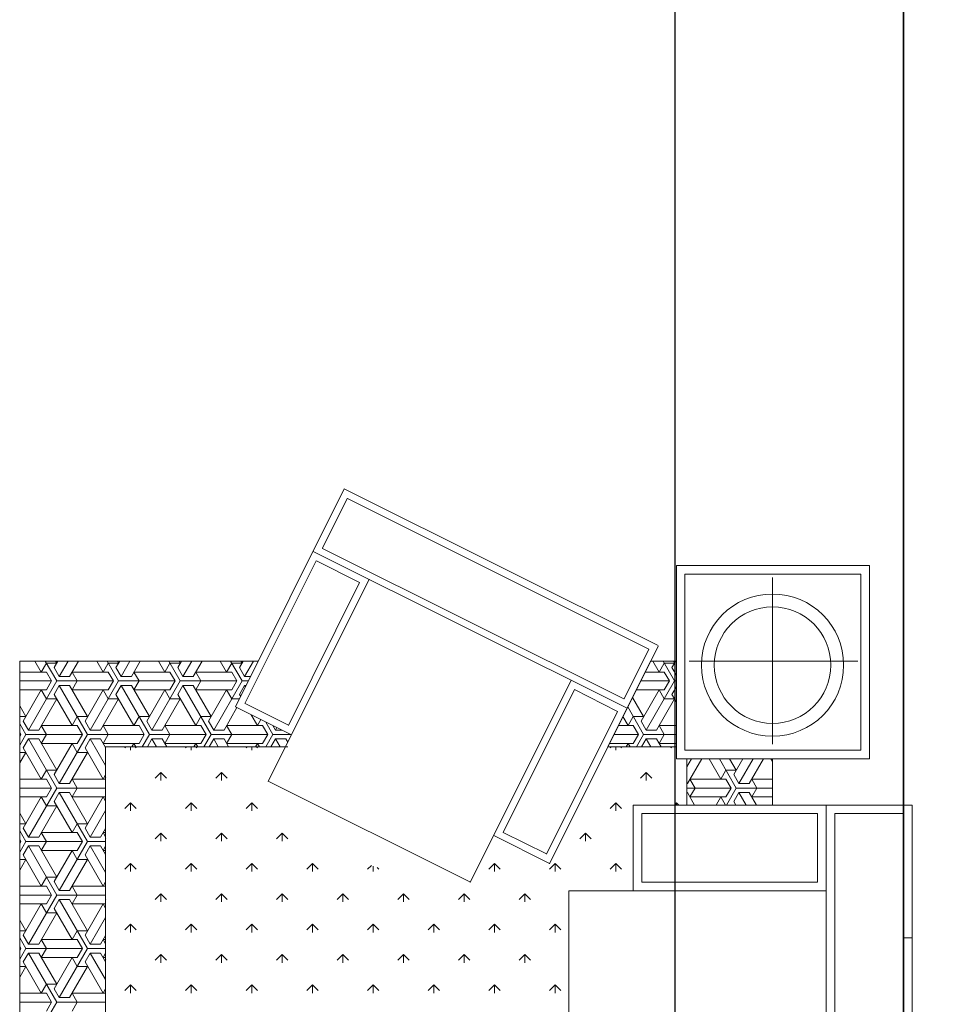
# Model space of a CAD drawing. Units: inches. Extents: x -1198 to -69, y -512 to 437.
# Tile 23 of 50: x -750 to -696, y 76 to 134. Entities that reach past the tile are written whole.
import ezdxf

# ---------------------------------------------------------------- set-up
doc = ezdxf.new("R2010")
doc.units = ezdxf.units.IN
doc.header["$MEASUREMENT"] = 0
for name, color, linetype, lineweight in [('A-ANNO-DIMS', 2, 'Continuous', 18), ('A-FURN', 60, 'Continuous', 18), ('A-WALL', 7, 'Continuous', 35), ('windows', 160, 'Continuous', 18)]:
    doc.layers.add(name, color=color, linetype=linetype, lineweight=lineweight)
doc.styles.get("Standard").update_dxf_attribs({"font": 'arial.ttf'})
doc.dimstyles.get("Standard").update_dxf_attribs({"dimtxt": 6, "dimasz": 6, "dimexe": 0.18, "dimexo": 0.0625, "dimgap": 0.09, "dimtad": 0, "dimtih": 1, "dimtoh": 1, "dimdec": 0, "dimzin": 0, "dimdsep": 46, "dimlunit": 4, "dimtxsty": 'Standard', "dimblk": 'OBLIQUE', "dimcen": 0.09, "dimadec": 0, "dimazin": 0, "dimtfac": 1, "dimtdec": 0, "dimtofl": 0, "dimtmove": 0, "dimatfit": 3, "dimfxl": 1, "dimtolj": 1, "dimtzin": 0, "dimarcsym": 0})

# ---------------------------------------------------------------- blocks, each defined once
blk = doc.blocks.new('A$C3B9F700E')
for p, q in [((736.9, 2080, -685.7), (2936.9, 2080, -685.7)), ((736.9, 2080, -685.7), (736.9, 1430, -685.7)), ((736.9, 1880, -685.7), (736.9, 2080, -685.7)), ((756.9, 2060, -685.7), (2916.9, 2060, -685.7)), ((756.9, 1900, -685.7), (756.9, 2060, -685.7)), ((179, 1980.6, -685.7), (179, 1530.6, -685.7)), ((629, 1980.6, -685.7), (179, 1980.6, -685.7)), ((629, 1530.6, -685.7), (629, 1980.6, -685.7)), ((199, 1960.6, -685.7), (199, 1550.6, -685.7)), ((609, 1960.6, -685.7), (199, 1960.6, -685.7)), ((401.3, 1953.9, -685.7), (401.3, 1560.5, -685.7)), ((609, 1550.6, -685.7), (609, 1960.6, -685.7)), ((2916.9, 1900, -685.7), (756.9, 1900, -685.7)), ((2936.9, 1880, -685.7), (736.9, 1880, -685.7)), ((2936.9, 1880, -685.7), (736.9, 1880, -685.7)), ((736.9, 1430, -685.7), (736.9, 1880, -685.7)), ((736.9, 1880, -685.7), (936.9, 1880, -685.7)), ((756.9, 1450, -685.7), (756.9, 1860, -685.7)), ((756.9, 1860, -685.7), (916.9, 1860, -685.7)), ((916.9, 1860, -685.7), (916.9, 1450, -685.7)), ((936.9, 1880, -685.7), (936.9, 1280, -685.7)), ((936.9, 1880, -685.7), (936.9, 1430, -685.7)), ((595.4, 1754.8, -685.7), (207.1, 1754.8, -685.7)), ((629, 1754.8, -685.7), (736.9, 1754.8, -685.7)), ((629, 1754.8, -685.7), (736.9, 1754.8, -685.7)), ((629, 1554.8, -685.7), (629, 1754.8, -685.7)), ((629, 1750.9, -685.7), (635.7, 1754.8, -685.7)), ((676.4, 1754.8, -685.7), (676.4, 1706.3, -685.7)), ((697.2, 1670.3, -685.7), (697.2, 1754.8, -685.7)), ((718, 1754.8, -685.7), (718, 1706.3, -685.7)), ((736.9, 1754.8, -685.7), (736.9, 1554.8, -685.7)), ((686.8, 1700.3, -685.7), (629, 1733.7, -685.7)), ((629, 1709.7, -685.7), (686.8, 1676.3, -685.7)), ((697.2, 1718.3, -685.7), (676.4, 1706.3, -685.7)), ((686.8, 1676.3, -685.7), (686.8, 1700.3, -685.7)), ((697.2, 1718.3, -685.7), (718, 1706.3, -685.7)), ((707.6, 1700.3, -685.7), (736.9, 1717.3, -685.7)), ((707.6, 1676.3, -685.7), (707.6, 1700.3, -685.7)), ((666, 1664.3, -685.7), (629, 1685.7, -685.7)), ((686.8, 1676.3, -685.7), (666, 1664.3, -685.7)), ((736.9, 1693.3, -685.7), (707.6, 1676.3, -685.7)), ((707.6, 1676.3, -685.7), (728.4, 1664.3, -685.7)), ((629, 1654.9, -685.7), (655.6, 1670.3, -685.7)), ((697.2, 1670.3, -685.7), (629, 1630.9, -685.7)), ((655.6, 1646.3, -685.7), (655.6, 1670.3, -685.7)), ((697.2, 1658.3, -685.7), (676.4, 1646.3, -685.7)), ((697.2, 1670.3, -685.7), (736.9, 1647.4, -685.7)), ((697.2, 1658.3, -685.7), (718, 1646.3, -685.7)), ((697.2, 1554.8, -685.7), (697.2, 1658.3, -685.7)), ((728.4, 1664.3, -685.7), (736.9, 1669.3, -685.7)), ((629, 1606.9, -685.7), (676.4, 1634.3, -685.7)), ((655.6, 1646.3, -685.7), (676.4, 1634.3, -685.7)), ((676.4, 1646.3, -685.7), (676.4, 1562.3, -685.7)), ((718, 1646.3, -685.7), (718, 1562.3, -685.7)), ((736.9, 1645.3, -685.7), (718, 1634.3, -685.7)), ((736.9, 1623.4, -685.7), (718, 1634.3, -685.7)), ((686.8, 1556.3, -685.7), (629, 1589.7, -685.7)), ((629, 1565.7, -685.7), (647.9, 1554.8, -685.7)), ((697.2, 1574.3, -685.7), (676.4, 1562.3, -685.7)), ((697.2, 1574.3, -685.7), (718, 1562.3, -685.7)), ((707.6, 1556.3, -685.7), (736.9, 1573.3, -685.7)), ((199, 1550.6, -685.7), (609, 1550.6, -685.7)), ((736.9, 1554.8, -685.7), (629, 1554.8, -685.7)), ((629, 1554.8, -685.7), (736.9, 1554.8, -685.7)), ((686.8, 1554.8, -685.7), (686.8, 1556.3, -685.7)), ((707.6, 1554.8, -685.7), (707.6, 1556.3, -685.7)), ((179, 1530.6, -685.7), (629, 1530.6, -685.7)), ((401.4, 1530.6, -685.7), (401.4, 1470.6, -685.7)), ((401.4, 1470.6, -685.7), (401.4, 1530.6, -685.7)), ((601.4, 1530.6, -685.7), (401.4, 1530.6, -685.7)), ((416.6, 1520.3, -685.7), (401.4, 1529.1, -685.7)), ((401.4, 1523.6, -685.7), (406.2, 1526.3, -685.7)), ((447.8, 1526.3, -685.7), (401.4, 1499.6, -685.7)), ((406.2, 1502.3, -685.7), (406.2, 1526.3, -685.7)), ((434.4, 1530.6, -685.7), (416.6, 1520.3, -685.7)), ((447.8, 1514.3, -685.7), (427, 1502.3, -685.7)), ((447.8, 1526.3, -685.7), (447.8, 1530.6, -685.7)), ((447.8, 1526.3, -685.7), (562.1, 1460.3, -685.7)), ((447.8, 1514.3, -685.7), (468.6, 1502.3, -685.7)), ((447.8, 1447.5, -685.7), (447.8, 1514.3, -685.7)), ((461.1, 1530.6, -685.7), (479, 1520.3, -685.7)), ((479, 1520.3, -685.7), (496.8, 1530.6, -685.7)), ((562.1, 1484.3, -685.7), (489.3, 1526.3, -685.7)), ((489.3, 1502.3, -685.7), (489.3, 1526.3, -685.7)), ((551.7, 1530.6, -685.7), (551.7, 1490.3, -685.7)), ((572.5, 1454.3, -685.7), (572.5, 1530.6, -685.7)), ((593.3, 1530.6, -685.7), (593.3, 1490.3, -685.7)), ((601.4, 1370.8, -685.7), (601.4, 1530.6, -685.7)), ((601.4, 1370.8, -685.7), (601.4, 1530.6, -685.7)), ((601.4, 1520.3, -685.7), (603.7, 1518, -685.7)), ((731.9, 1531.3, -685.7), (736.9, 1536.3, -685.7)), ((731.9, 1531.3, -685.7), (736.9, 1526.2, -685.7)), ((731.9, 1531.3, -685.7), (736.9, 1531.3, -685.7)), ((406.2, 1502.3, -685.7), (427, 1490.3, -685.7)), ((427, 1502.3, -685.7), (427, 1457.9, -685.7)), ((468.6, 1502.3, -685.7), (468.6, 1437.1, -685.7)), ((489.3, 1502.3, -685.7), (468.6, 1490.3, -685.7)), ((572.5, 1502.3, -685.7), (551.7, 1490.3, -685.7)), ((572.5, 1502.3, -685.7), (593.3, 1490.3, -685.7)), ((582.9, 1484.3, -685.7), (601.4, 1495, -685.7)), ((365.5, 1488.6, -685.7), (0, 756.7, -685.7)), ((873.7, 1234.8, -685.7), (366.4, 1488.1, -685.7)), ((401.4, 1475.6, -685.7), (427, 1490.3, -685.7)), ((401.4, 1470.6, -685.7), (601.4, 1370.8, -685.7)), ((541.3, 1448.3, -685.7), (468.6, 1490.3, -685.7)), ((562.1, 1460.3, -685.7), (562.1, 1484.3, -685.7)), ((582.9, 1460.3, -685.7), (582.9, 1484.3, -685.7)), ((601.4, 1471, -685.7), (582.9, 1460.3, -685.7)), ((661.2, 1460.6, -685.7), (674.4, 1473.8, -685.7)), ((373.6, 1466.4, -685.7), (22.8, 763.8, -685.7)), ((489.2, 1408.7, -685.7), (373.6, 1466.4, -685.7)), ((486, 1428.4, -685.7), (530.9, 1454.3, -685.7)), ((572.5, 1454.3, -685.7), (508.3, 1417.3, -685.7)), ((530.9, 1430.3, -685.7), (530.9, 1454.3, -685.7)), ((562.1, 1460.3, -685.7), (541.3, 1448.3, -685.7)), ((572.5, 1454.3, -685.7), (601.4, 1437.6, -685.7)), ((582.9, 1460.3, -685.7), (601.4, 1449.6, -685.7)), ((661.2, 1460.6, -685.7), (674.4, 1447.3, -685.7)), ((661.2, 1460.6, -685.7), (679.9, 1460.6, -685.7)), ((916.9, 1450, -685.7), (756.9, 1450, -685.7)), ((530.9, 1430.3, -685.7), (551.7, 1418.3, -685.7)), ((572.5, 1442.3, -685.7), (551.7, 1430.3, -685.7)), ((551.7, 1430.3, -685.7), (551.7, 1395.6, -685.7)), ((572.5, 1385.2, -685.7), (572.5, 1442.3, -685.7)), ((572.5, 1442.3, -685.7), (593.3, 1430.3, -685.7)), ((593.3, 1430.3, -685.7), (593.3, 1374.8, -685.7)), ((601.4, 1423, -685.7), (593.3, 1418.3, -685.7)), ((936.9, 1430, -685.7), (736.9, 1430, -685.7)), ((138.8, 705.9, -685.7), (489.4, 1408.1, -685.7)), ((511.3, 1415.8, -685.7), (145.8, 683.8, -685.7)), ((489.4, 1408.1, -685.7), (489.2, 1408.7, -685.7)), ((530.6, 1406.1, -685.7), (551.7, 1418.3, -685.7)), ((601.4, 1413.6, -685.7), (593.3, 1418.3, -685.7)), ((601.4, 1400.9, -685.7), (603.7, 1403.1, -685.7)), ((731.9, 1389.9, -685.7), (745.1, 1403.1, -685.7)), ((873.3, 1389.9, -685.7), (886.5, 1403.1, -685.7)), ((518.9, 1393.8, -685.7), (467.6, 1293.2, -685.7)), ((851.6, 1227.8, -685.7), (518.9, 1393.8, -685.7)), ((601.4, 1389.9, -685.7), (609.2, 1389.9, -685.7)), ((601.4, 1378.9, -685.7), (603.7, 1376.6, -685.7)), ((731.9, 1389.9, -685.7), (750.6, 1389.9, -685.7)), ((731.9, 1389.9, -685.7), (745.1, 1376.6, -685.7)), ((873.3, 1389.9, -685.7), (892, 1389.9, -685.7)), ((873.3, 1389.9, -685.7), (886.5, 1376.6, -685.7)), ((802.6, 1319.2, -685.7), (815.8, 1332.4, -685.7)), ((802.6, 1319.2, -685.7), (815.8, 1305.9, -685.7)), ((802.6, 1319.2, -685.7), (821.3, 1319.2, -685.7)), ((917.2, 1050.1, -685.7), (446.2, 1285.3, -685.7)), ((800.5, 1126.9, -685.7), (467.6, 1293.2, -685.7)), ((2736.9, 1280, -685.7), (936.9, 1280, -685.7)), ((873.3, 1248.4, -685.7), (886.5, 1261.7, -685.7)), ((873.3, 1248.4, -685.7), (886.5, 1235.2, -685.7)), ((873.3, 1248.4, -685.7), (892, 1248.4, -685.7)), ((1014.7, 1248.4, -685.7), (1028, 1261.7, -685.7)), ((1014.7, 1248.4, -685.7), (1028, 1235.2, -685.7)), ((1014.7, 1248.4, -685.7), (1033.5, 1248.4, -685.7)), ((1156.1, 1248.4, -685.7), (1169.4, 1261.7, -685.7)), ((1156.1, 1248.4, -685.7), (1169.4, 1235.2, -685.7)), ((1156.1, 1248.4, -685.7), (1174.9, 1248.4, -685.7)), ((850.8, 1227.7, -685.7), (800.5, 1126.9, -685.7)), ((872.8, 1235.3, -685.7), (807.6, 1104.8, -685.7)), ((944, 1177.7, -685.7), (957.3, 1191, -685.7)), ((944, 1177.7, -685.7), (957.3, 1164.5, -685.7)), ((944, 1177.7, -685.7), (962.7, 1177.7, -685.7)), ((1085.4, 1177.7, -685.7), (1098.7, 1191, -685.7)), ((1085.4, 1177.7, -685.7), (1098.7, 1164.5, -685.7)), ((1085.4, 1177.7, -685.7), (1104.2, 1177.7, -685.7)), ((873.3, 1107, -685.7), (886.5, 1120.3, -685.7)), ((873.3, 1107, -685.7), (886.5, 1093.8, -685.7)), ((873.3, 1107, -685.7), (892, 1107, -685.7)), ((1014.7, 1107, -685.7), (1028, 1120.3, -685.7)), ((1014.7, 1107, -685.7), (1028, 1093.8, -685.7)), ((1014.7, 1107, -685.7), (1033.5, 1107, -685.7)), ((1156.1, 1107, -685.7), (1169.4, 1120.3, -685.7)), ((1156.1, 1107, -685.7), (1169.4, 1093.8, -685.7)), ((1156.1, 1107, -685.7), (1174.9, 1107, -685.7)), ((916.3, 1050.6, -685.7), (681.1, 579.5, -685.7)), ((944, 1036.3, -685.7), (957.3, 1049.6, -685.7)), ((944, 1036.3, -685.7), (957.3, 1023.1, -685.7)), ((944, 1036.3, -685.7), (962.7, 1036.3, -685.7)), ((1085.4, 1036.3, -685.7), (1098.7, 1049.6, -685.7)), ((1085.4, 1036.3, -685.7), (1098.7, 1023.1, -685.7)), ((1085.4, 1036.3, -685.7), (1104.2, 1036.3, -685.7)), ((1014.7, 965.6, -685.7), (1028, 978.9, -685.7)), ((1014.7, 965.6, -685.7), (1028, 952.3, -685.7)), ((1014.7, 965.6, -685.7), (1033.5, 965.6, -685.7)), ((1156.1, 965.6, -685.7), (1169.4, 978.9, -685.7)), ((1156.1, 965.6, -685.7), (1169.4, 952.3, -685.7)), ((1156.1, 965.6, -685.7), (1174.9, 965.6, -685.7)), ((944, 894.9, -685.7), (957.3, 908.1, -685.7)), ((944, 894.9, -685.7), (957.3, 881.6, -685.7)), ((944, 894.9, -685.7), (962.7, 894.9, -685.7)), ((1085.4, 894.9, -685.7), (1098.7, 908.1, -685.7)), ((1085.4, 894.9, -685.7), (1098.7, 881.6, -685.7)), ((1085.4, 894.9, -685.7), (1104.2, 894.9, -685.7)), ((882.6, 833.5, -685.7), (886.5, 837.4, -685.7)), ((1014.7, 824.2, -685.7), (1028, 837.4, -685.7)), ((1156.1, 824.2, -685.7), (1169.4, 837.4, -685.7)), ((682, 579.1, -685.7), (211, 814.3, -685.7)), ((877.8, 819.7, -685.7), (886.5, 810.9, -685.7)), ((879.4, 824.2, -685.7), (892, 824.2, -685.7)), ((1014.7, 824.2, -685.7), (1028, 810.9, -685.7)), ((1014.7, 824.2, -685.7), (1033.5, 824.2, -685.7)), ((1156.1, 824.2, -685.7), (1169.4, 810.9, -685.7)), ((1156.1, 824.2, -685.7), (1174.9, 824.2, -685.7)), ((218.1, 792.2, -685.7), (167.8, 691.5, -685.7)), ((551.2, 626.3, -685.7), (218.6, 792.4, -685.7)), ((22.8, 763.8, -685.7), (23, 763.3, -685.7)), ((23, 763.3, -685.7), (138.2, 705.7, -685.7)), ((944, 753.5, -685.7), (957.3, 766.7, -685.7)), ((1085.4, 753.5, -685.7), (1098.7, 766.7, -685.7)), ((508.2, 502.9, -685.7), (0, 756.7, -685.7)), ((944, 753.5, -685.7), (957.3, 740.2, -685.7)), ((944, 753.5, -685.7), (962.7, 753.5, -685.7)), ((1085.4, 753.5, -685.7), (1098.7, 740.2, -685.7)), ((1085.4, 753.5, -685.7), (1104.2, 753.5, -685.7)), ((138.2, 705.7, -685.7), (138.8, 705.9, -685.7)), ((500.6, 524.8, -685.7), (167.9, 690.9, -685.7)), ((873.3, 682.8, -685.7), (886.5, 696, -685.7)), ((1014.7, 682.8, -685.7), (1028, 696, -685.7)), ((1156.1, 682.8, -685.7), (1169.4, 696, -685.7)), ((873.3, 682.8, -685.7), (886.5, 669.5, -685.7)), ((873.3, 682.8, -685.7), (892, 682.8, -685.7)), ((1014.7, 682.8, -685.7), (1028, 669.5, -685.7)), ((1014.7, 682.8, -685.7), (1033.5, 682.8, -685.7)), ((1156.1, 682.8, -685.7), (1169.4, 669.5, -685.7)), ((1156.1, 682.8, -685.7), (1174.9, 682.8, -685.7)), ((550.5, 626.2, -685.7), (500.2, 525.5, -685.7)), ((573.3, 633.3, -685.7), (508.2, 502.9, -685.7)), ((573.3, 633.3, -685.7), (508.2, 502.9, -685.7)), ((572.5, 590.3, -685.7), (572.5, 631.7, -685.7)), ((601.4, 619.3, -685.7), (573.3, 633.3, -685.7)), ((582.9, 620.3, -685.7), (590.5, 624.7, -685.7)), ((582.9, 596.3, -685.7), (582.9, 620.3, -685.7)), ((601.4, 200, -685.7), (601.4, 624.9, -685.7)), ((802.6, 612, -685.7), (815.8, 625.3, -685.7)), ((944, 612, -685.7), (957.3, 625.3, -685.7)), ((1085.4, 612, -685.7), (1098.7, 625.3, -685.7)), ((556.5, 599.6, -685.7), (562.1, 596.3, -685.7)), ((562.1, 596.3, -685.7), (562.1, 610.8, -685.7)), ((601.4, 607, -685.7), (582.9, 596.3, -685.7)), ((601.4, 200, -685.7), (601.4, 619.3, -685.7)), ((802.6, 612, -685.7), (815.8, 598.8, -685.7)), ((802.6, 612, -685.7), (821.3, 612, -685.7)), ((944, 612, -685.7), (957.3, 598.8, -685.7)), ((944, 612, -685.7), (962.7, 612, -685.7)), ((1085.4, 612, -685.7), (1098.7, 598.8, -685.7)), ((1085.4, 612, -685.7), (1104.2, 612, -685.7)), ((572.5, 590.3, -685.7), (543.5, 573.6, -685.7)), ((572.5, 578.3, -685.7), (551.7, 566.3, -685.7)), ((562.1, 596.3, -685.7), (551.9, 590.4, -685.7)), ((572.5, 590.3, -685.7), (601.4, 573.6, -685.7)), ((572.5, 578.3, -685.7), (593.3, 566.3, -685.7)), ((572.5, 446.3, -685.7), (572.5, 578.3, -685.7)), ((582.9, 596.3, -685.7), (601.4, 585.6, -685.7)), ((401.4, 556.2, -685.7), (401.4, 0, -685.7)), ((508.2, 502.9, -685.7), (401.4, 556.2, -685.7)), ((401.4, 0, -685.7), (401.4, 556.2, -685.7)), ((526.6, 539.9, -685.7), (551.7, 554.3, -685.7)), ((537.9, 562.3, -685.7), (551.7, 554.3, -685.7)), ((551.7, 566.3, -685.7), (551.7, 482.3, -685.7)), ((593.3, 566.3, -685.7), (593.3, 482.3, -685.7)), ((601.4, 559, -685.7), (593.3, 554.3, -685.7)), ((601.4, 549.6, -685.7), (593.3, 554.3, -685.7)), ((601.4, 552.3, -685.7), (603.7, 554.6, -685.7)), ((731.9, 541.3, -685.7), (745.1, 554.6, -685.7)), ((873.3, 541.3, -685.7), (886.5, 554.6, -685.7)), ((1014.7, 541.3, -685.7), (1028, 554.6, -685.7)), ((1156.1, 541.3, -685.7), (1169.4, 554.6, -685.7)), ((401.4, 545.1, -685.7), (437.4, 524.3, -685.7)), ((437.4, 524.3, -685.7), (437.4, 538.3, -685.7)), ((447.8, 518.3, -685.7), (447.8, 533.1, -685.7)), ((458.2, 524.3, -685.7), (458.2, 527.9, -685.7)), ((601.4, 541.3, -685.7), (609.2, 541.3, -685.7)), ((601.4, 530.3, -685.7), (603.7, 528.1, -685.7)), ((731.9, 541.3, -685.7), (745.1, 528.1, -685.7)), ((731.9, 541.3, -685.7), (750.6, 541.3, -685.7)), ((873.3, 541.3, -685.7), (886.5, 528.1, -685.7)), ((873.3, 541.3, -685.7), (892, 541.3, -685.7)), ((1014.7, 541.3, -685.7), (1028, 528.1, -685.7)), ((1014.7, 541.3, -685.7), (1033.5, 541.3, -685.7)), ((1156.1, 541.3, -685.7), (1169.4, 528.1, -685.7)), ((1156.1, 541.3, -685.7), (1174.9, 541.3, -685.7)), ((416.6, 512.3, -685.7), (401.4, 521.1, -685.7)), ((401.4, 515.6, -685.7), (406.2, 518.3, -685.7)), ((447.8, 518.3, -685.7), (401.4, 491.6, -685.7)), ((406.2, 494.3, -685.7), (406.2, 518.3, -685.7)), ((437.4, 524.3, -685.7), (416.6, 512.3, -685.7)), ((447.8, 506.3, -685.7), (427, 494.3, -685.7)), ((447.8, 518.3, -685.7), (562.1, 452.3, -685.7)), ((447.8, 506.3, -685.7), (468.6, 494.3, -685.7)), ((447.8, 374.3, -685.7), (447.8, 506.3, -685.7)), ((461.5, 526.2, -685.7), (458.2, 524.3, -685.7)), ((458.2, 524.3, -685.7), (479, 512.3, -685.7)), ((479, 512.3, -685.7), (483.8, 515.1, -685.7)), ((489.3, 494.3, -685.7), (489.3, 512.3, -685.7)), ((562.1, 476.3, -685.7), (509.9, 506.4, -685.7)), ((401.4, 467.6, -685.7), (427, 482.3, -685.7)), ((406.2, 494.3, -685.7), (427, 482.3, -685.7)), ((427, 494.3, -685.7), (427, 410.3, -685.7)), ((468.6, 494.3, -685.7), (468.6, 410.3, -685.7)), ((489.3, 494.3, -685.7), (468.6, 482.3, -685.7)), ((541.3, 440.3, -685.7), (468.6, 482.3, -685.7)), ((572.5, 494.3, -685.7), (551.7, 482.3, -685.7)), ((572.5, 494.3, -685.7), (593.3, 482.3, -685.7)), ((582.9, 476.3, -685.7), (601.4, 487, -685.7)), ((661.2, 470.6, -685.7), (674.4, 483.9, -685.7)), ((802.6, 470.6, -685.7), (815.8, 483.9, -685.7)), ((944, 470.6, -685.7), (957.3, 483.9, -685.7)), ((1085.4, 470.6, -685.7), (1098.7, 483.9, -685.7)), ((562.1, 452.3, -685.7), (562.1, 476.3, -685.7)), ((582.9, 452.3, -685.7), (582.9, 476.3, -685.7)), ((601.4, 463, -685.7), (582.9, 452.3, -685.7)), ((661.2, 470.6, -685.7), (679.9, 470.6, -685.7)), ((661.2, 470.6, -685.7), (674.4, 457.4, -685.7)), ((802.6, 470.6, -685.7), (821.3, 470.6, -685.7)), ((802.6, 470.6, -685.7), (815.8, 457.4, -685.7)), ((944, 470.6, -685.7), (962.7, 470.6, -685.7)), ((944, 470.6, -685.7), (957.3, 457.4, -685.7)), ((1085.4, 470.6, -685.7), (1104.2, 470.6, -685.7)), ((1085.4, 470.6, -685.7), (1098.7, 457.4, -685.7)), ((458.2, 404.3, -685.7), (530.9, 446.3, -685.7)), ((572.5, 446.3, -685.7), (458.2, 380.3, -685.7)), ((530.9, 422.3, -685.7), (530.9, 446.3, -685.7)), ((562.1, 452.3, -685.7), (541.3, 440.3, -685.7)), ((572.5, 446.3, -685.7), (601.4, 429.6, -685.7)), ((582.9, 452.3, -685.7), (601.4, 441.6, -685.7)), ((437.4, 404.3, -685.7), (401.4, 425.1, -685.7)), ((447.8, 422.3, -685.7), (427, 410.3, -685.7)), ((447.8, 422.3, -685.7), (468.6, 410.3, -685.7)), ((530.9, 422.3, -685.7), (551.7, 410.3, -685.7)), ((572.5, 434.3, -685.7), (551.7, 422.3, -685.7)), ((551.7, 422.3, -685.7), (551.7, 338.3, -685.7)), ((572.5, 434.3, -685.7), (593.3, 422.3, -685.7)), ((572.5, 302.3, -685.7), (572.5, 434.3, -685.7)), ((593.3, 422.3, -685.7), (593.3, 338.3, -685.7)), ((601.4, 415, -685.7), (593.3, 410.3, -685.7)), ((601.4, 410.9, -685.7), (603.7, 413.2, -685.7)), ((731.9, 399.9, -685.7), (745.1, 413.2, -685.7)), ((873.3, 399.9, -685.7), (886.5, 413.2, -685.7)), ((1014.7, 399.9, -685.7), (1028, 413.2, -685.7)), ((1156.1, 399.9, -685.7), (1169.4, 413.2, -685.7)), ((401.4, 401.1, -685.7), (437.4, 380.3, -685.7)), ((437.4, 380.3, -685.7), (437.4, 404.3, -685.7)), ((458.2, 380.3, -685.7), (458.2, 404.3, -685.7)), ((479, 368.3, -685.7), (551.7, 410.3, -685.7)), ((601.4, 405.6, -685.7), (593.3, 410.3, -685.7)), ((601.4, 399.9, -685.7), (609.2, 399.9, -685.7)), ((731.9, 399.9, -685.7), (750.6, 399.9, -685.7)), ((731.9, 399.9, -685.7), (745.1, 386.7, -685.7)), ((873.3, 399.9, -685.7), (892, 399.9, -685.7)), ((873.3, 399.9, -685.7), (886.5, 386.7, -685.7)), ((1014.7, 399.9, -685.7), (1033.5, 399.9, -685.7)), ((1014.7, 399.9, -685.7), (1028, 386.7, -685.7)), ((1156.1, 399.9, -685.7), (1174.9, 399.9, -685.7)), ((1156.1, 399.9, -685.7), (1169.4, 386.7, -685.7)), ((416.6, 368.3, -685.7), (401.4, 377.1, -685.7)), ((401.4, 371.6, -685.7), (406.2, 374.3, -685.7)), ((447.8, 374.3, -685.7), (401.4, 347.6, -685.7)), ((406.2, 350.3, -685.7), (406.2, 374.3, -685.7)), ((437.4, 380.3, -685.7), (416.6, 368.3, -685.7)), ((447.8, 374.3, -685.7), (562.1, 308.3, -685.7)), ((458.2, 380.3, -685.7), (479, 368.3, -685.7)), ((562.1, 332.3, -685.7), (489.3, 374.3, -685.7)), ((489.3, 350.3, -685.7), (489.3, 374.3, -685.7)), ((601.4, 388.9, -685.7), (603.7, 386.7, -685.7)), ((406.2, 350.3, -685.7), (427, 338.3, -685.7)), ((447.8, 362.3, -685.7), (427, 350.3, -685.7)), ((427, 350.3, -685.7), (427, 266.3, -685.7)), ((447.8, 362.3, -685.7), (468.6, 350.3, -685.7)), ((447.8, 230.3, -685.7), (447.8, 362.3, -685.7)), ((468.6, 350.3, -685.7), (468.6, 266.3, -685.7)), ((489.3, 350.3, -685.7), (468.6, 338.3, -685.7)), ((572.5, 350.3, -685.7), (551.7, 338.3, -685.7)), ((572.5, 350.3, -685.7), (593.3, 338.3, -685.7)), ((401.4, 323.6, -685.7), (427, 338.3, -685.7)), ((541.3, 296.3, -685.7), (468.6, 338.3, -685.7)), ((562.1, 308.3, -685.7), (562.1, 332.3, -685.7)), ((582.9, 332.3, -685.7), (601.4, 343, -685.7)), ((582.9, 308.3, -685.7), (582.9, 332.3, -685.7)), ((661.2, 329.2, -685.7), (674.4, 342.5, -685.7)), ((661.2, 329.2, -685.7), (674.4, 315.9, -685.7)), ((661.2, 329.2, -685.7), (679.9, 329.2, -685.7)), ((802.6, 329.2, -685.7), (815.8, 342.5, -685.7)), ((802.6, 329.2, -685.7), (815.8, 315.9, -685.7)), ((802.6, 329.2, -685.7), (821.3, 329.2, -685.7)), ((944, 329.2, -685.7), (957.3, 342.5, -685.7)), ((944, 329.2, -685.7), (957.3, 315.9, -685.7)), ((944, 329.2, -685.7), (962.7, 329.2, -685.7)), ((1085.4, 329.2, -685.7), (1098.7, 342.5, -685.7)), ((1085.4, 329.2, -685.7), (1098.7, 315.9, -685.7)), ((1085.4, 329.2, -685.7), (1104.2, 329.2, -685.7)), ((458.2, 260.3, -685.7), (530.9, 302.3, -685.7)), ((572.5, 302.3, -685.7), (458.2, 236.3, -685.7)), ((530.9, 278.3, -685.7), (530.9, 302.3, -685.7)), ((562.1, 308.3, -685.7), (541.3, 296.3, -685.7)), ((572.5, 302.3, -685.7), (601.4, 285.6, -685.7)), ((601.4, 319, -685.7), (582.9, 308.3, -685.7)), ((582.9, 308.3, -685.7), (601.4, 297.6, -685.7)), ((437.4, 260.3, -685.7), (401.4, 281.1, -685.7)), ((447.8, 278.3, -685.7), (427, 266.3, -685.7)), ((447.8, 278.3, -685.7), (468.6, 266.3, -685.7)), ((530.9, 278.3, -685.7), (551.7, 266.3, -685.7)), ((572.5, 290.3, -685.7), (551.7, 278.3, -685.7)), ((551.7, 278.3, -685.7), (551.7, 194.3, -685.7)), ((572.5, 290.3, -685.7), (593.3, 278.3, -685.7)), ((572.5, 158.3, -685.7), (572.5, 290.3, -685.7)), ((593.3, 278.3, -685.7), (593.3, 194.3, -685.7)), ((401.4, 257.1, -685.7), (437.4, 236.3, -685.7)), ((437.4, 236.3, -685.7), (437.4, 260.3, -685.7)), ((458.2, 236.3, -685.7), (458.2, 260.3, -685.7)), ((479, 224.3, -685.7), (551.7, 266.3, -685.7)), ((601.4, 271, -685.7), (593.3, 266.3, -685.7)), ((601.4, 261.6, -685.7), (593.3, 266.3, -685.7)), ((601.4, 269.5, -685.7), (603.7, 271.8, -685.7)), ((601.4, 258.5, -685.7), (609.2, 258.5, -685.7)), ((731.9, 258.5, -685.7), (745.1, 271.8, -685.7)), ((731.9, 258.5, -685.7), (745.1, 245.2, -685.7)), ((731.9, 258.5, -685.7), (750.6, 258.5, -685.7)), ((873.3, 258.5, -685.7), (886.5, 271.8, -685.7)), ((873.3, 258.5, -685.7), (886.5, 245.2, -685.7)), ((873.3, 258.5, -685.7), (892, 258.5, -685.7)), ((1014.7, 258.5, -685.7), (1028, 271.8, -685.7)), ((1014.7, 258.5, -685.7), (1028, 245.2, -685.7)), ((1014.7, 258.5, -685.7), (1033.5, 258.5, -685.7)), ((1156.1, 258.5, -685.7), (1169.4, 271.8, -685.7)), ((1156.1, 258.5, -685.7), (1169.4, 245.2, -685.7)), ((1156.1, 258.5, -685.7), (1174.9, 258.5, -685.7)), ((416.6, 224.3, -685.7), (401.4, 233.1, -685.7)), ((401.4, 227.6, -685.7), (406.2, 230.3, -685.7)), ((447.8, 230.3, -685.7), (401.4, 203.6, -685.7)), ((406.2, 206.3, -685.7), (406.2, 230.3, -685.7)), ((437.4, 236.3, -685.7), (416.6, 224.3, -685.7)), ((447.8, 230.3, -685.7), (562.1, 164.3, -685.7)), ((458.2, 236.3, -685.7), (479, 224.3, -685.7)), ((562.1, 188.3, -685.7), (489.3, 230.3, -685.7)), ((489.3, 206.3, -685.7), (489.3, 230.3, -685.7)), ((601.4, 247.5, -685.7), (603.7, 245.2, -685.7)), ((447.8, 218.3, -685.7), (427, 206.3, -685.7)), ((447.8, 218.3, -685.7), (468.6, 206.3, -685.7)), ((447.8, 86.3, -685.7), (447.8, 218.3, -685.7)), ((401.4, 179.6, -685.7), (427, 194.3, -685.7)), ((406.2, 206.3, -685.7), (427, 194.3, -685.7)), ((427, 206.3, -685.7), (427, 122.3, -685.7)), ((468.6, 206.3, -685.7), (468.6, 122.3, -685.7)), ((489.3, 206.3, -685.7), (468.6, 194.3, -685.7)), ((541.3, 152.3, -685.7), (468.6, 194.3, -685.7)), ((572.5, 206.3, -685.7), (551.7, 194.3, -685.7)), ((562.1, 164.3, -685.7), (562.1, 188.3, -685.7)), ((572.5, 206.3, -685.7), (593.3, 194.3, -685.7)), ((582.9, 188.3, -685.7), (603.1, 200, -685.7)), ((644.7, 200, -685.7), (582.9, 164.3, -685.7)), ((582.9, 164.3, -685.7), (582.9, 188.3, -685.7)), ((3062.1, 200, -685.7), (601.4, 200, -685.7)), ((3062.1, 200, -685.7), (601.4, 200, -685.7)), ((603.7, 152.3, -685.7), (676.4, 194.3, -685.7)), ((666.6, 200, -685.7), (676.4, 194.3, -685.7)), ((673.4, 200, -685.7), (674.4, 201, -685.7)), ((676.4, 200, -685.7), (676.4, 122.3, -685.7)), ((697.2, 86.3, -685.7), (697.2, 200, -685.7)), ((718, 200, -685.7), (718, 122.3, -685.7)), ((727.8, 200, -685.7), (718, 194.3, -685.7)), ((790.7, 152.3, -685.7), (718, 194.3, -685.7)), ((749.7, 200, -685.7), (811.5, 164.3, -685.7)), ((811.5, 188.3, -685.7), (791.3, 200, -685.7)), ((801.1, 200, -685.7), (801.1, 194.3, -685.7)), ((811, 200, -685.7), (801.1, 194.3, -685.7)), ((811.5, 164.3, -685.7), (811.5, 188.3, -685.7)), ((814.8, 200, -685.7), (815.8, 201, -685.7)), ((821.9, 158.3, -685.7), (821.9, 200, -685.7)), ((832.3, 188.3, -685.7), (852.5, 200, -685.7)), ((894.1, 200, -685.7), (832.3, 164.3, -685.7)), ((832.3, 164.3, -685.7), (832.3, 188.3, -685.7)), ((832.8, 200, -685.7), (842.7, 194.3, -685.7)), ((842.7, 200, -685.7), (842.7, 194.3, -685.7)), ((853.1, 152.3, -685.7), (925.8, 194.3, -685.7)), ((916, 200, -685.7), (925.8, 194.3, -685.7)), ((925.8, 200, -685.7), (925.8, 122.3, -685.7)), ((946.6, 86.3, -685.7), (946.6, 200, -685.7)), ((956.2, 200, -685.7), (957.3, 201, -685.7)), ((967.4, 200, -685.7), (967.4, 122.3, -685.7)), ((977.2, 200, -685.7), (967.4, 194.3, -685.7)), ((1040.1, 152.3, -685.7), (967.4, 194.3, -685.7)), ((999.1, 200, -685.7), (1060.9, 164.3, -685.7)), ((1060.9, 188.3, -685.7), (1040.7, 200, -685.7)), ((1050.5, 200, -685.7), (1050.5, 194.3, -685.7)), ((1060.4, 200, -685.7), (1050.5, 194.3, -685.7)), ((1060.9, 164.3, -685.7), (1060.9, 188.3, -685.7)), ((1071.3, 158.3, -685.7), (1071.3, 200, -685.7)), ((1081.7, 188.3, -685.7), (1101.9, 200, -685.7)), ((1143.5, 200, -685.7), (1081.7, 164.3, -685.7)), ((1081.7, 164.3, -685.7), (1081.7, 188.3, -685.7)), ((1082.3, 200, -685.7), (1092.1, 194.3, -685.7)), ((1092.1, 200, -685.7), (1092.1, 194.3, -685.7)), ((1097.6, 200, -685.7), (1098.7, 201, -685.7)), ((1102.5, 152.3, -685.7), (1175.2, 194.3, -685.7)), ((1165.4, 200, -685.7), (1175.2, 194.3, -685.7)), ((1175.2, 200, -685.7), (1175.2, 122.3, -685.7)), ((1196, 86.3, -685.7), (1196, 200, -685.7)), ((562.1, 164.3, -685.7), (541.3, 152.3, -685.7)), ((582.9, 164.3, -685.7), (603.7, 152.3, -685.7)), ((811.5, 164.3, -685.7), (790.7, 152.3, -685.7)), ((832.3, 164.3, -685.7), (853.1, 152.3, -685.7)), ((1060.9, 164.3, -685.7), (1040.1, 152.3, -685.7)), ((1081.7, 164.3, -685.7), (1102.5, 152.3, -685.7)), ((458.2, 116.3, -685.7), (530.9, 158.3, -685.7)), ((572.5, 158.3, -685.7), (458.2, 92.3, -685.7)), ((530.9, 134.3, -685.7), (530.9, 158.3, -685.7)), ((572.5, 146.3, -685.7), (551.7, 134.3, -685.7)), ((572.5, 158.3, -685.7), (686.8, 92.3, -685.7)), ((572.5, 146.3, -685.7), (593.3, 134.3, -685.7)), ((572.5, 14.3, -685.7), (572.5, 146.3, -685.7)), ((686.8, 116.3, -685.7), (614.1, 158.3, -685.7)), ((614.1, 134.3, -685.7), (614.1, 158.3, -685.7)), ((707.6, 116.3, -685.7), (780.3, 158.3, -685.7)), ((821.9, 158.3, -685.7), (707.6, 92.3, -685.7)), ((780.3, 134.3, -685.7), (780.3, 158.3, -685.7)), ((821.9, 146.3, -685.7), (801.1, 134.3, -685.7)), ((821.9, 158.3, -685.7), (936.2, 92.3, -685.7)), ((821.9, 146.3, -685.7), (842.7, 134.3, -685.7)), ((821.9, 14.3, -685.7), (821.9, 146.3, -685.7)), ((936.2, 116.3, -685.7), (863.5, 158.3, -685.7)), ((863.5, 134.3, -685.7), (863.5, 158.3, -685.7)), ((957, 116.3, -685.7), (1029.7, 158.3, -685.7)), ((1071.3, 158.3, -685.7), (957, 92.3, -685.7)), ((1029.7, 134.3, -685.7), (1029.7, 158.3, -685.7)), ((1071.3, 146.3, -685.7), (1050.5, 134.3, -685.7)), ((1071.3, 158.3, -685.7), (1185.6, 92.3, -685.7)), ((1071.3, 146.3, -685.7), (1092.1, 134.3, -685.7)), ((1071.3, 14.3, -685.7), (1071.3, 146.3, -685.7)), ((1185.6, 116.3, -685.7), (1112.9, 158.3, -685.7)), ((1112.9, 134.3, -685.7), (1112.9, 158.3, -685.7)), ((437.4, 116.3, -685.7), (401.4, 137.1, -685.7)), ((447.8, 134.3, -685.7), (427, 122.3, -685.7)), ((437.4, 92.3, -685.7), (437.4, 116.3, -685.7)), ((447.8, 134.3, -685.7), (468.6, 122.3, -685.7)), ((458.2, 92.3, -685.7), (458.2, 116.3, -685.7)), ((479, 80.3, -685.7), (551.7, 122.3, -685.7)), ((530.9, 134.3, -685.7), (551.7, 122.3, -685.7)), ((551.7, 134.3, -685.7), (551.7, 50.3, -685.7)), ((593.3, 134.3, -685.7), (593.3, 50.3, -685.7)), ((614.1, 134.3, -685.7), (593.3, 122.3, -685.7)), ((666, 80.3, -685.7), (593.3, 122.3, -685.7)), ((697.2, 134.3, -685.7), (676.4, 122.3, -685.7)), ((686.8, 92.3, -685.7), (686.8, 116.3, -685.7)), ((697.2, 134.3, -685.7), (718, 122.3, -685.7)), ((707.6, 92.3, -685.7), (707.6, 116.3, -685.7)), ((728.4, 80.3, -685.7), (801.1, 122.3, -685.7)), ((780.3, 134.3, -685.7), (801.1, 122.3, -685.7)), ((801.1, 134.3, -685.7), (801.1, 50.3, -685.7)), ((842.7, 134.3, -685.7), (842.7, 50.3, -685.7)), ((863.5, 134.3, -685.7), (842.7, 122.3, -685.7)), ((915.4, 80.3, -685.7), (842.7, 122.3, -685.7)), ((946.6, 134.3, -685.7), (925.8, 122.3, -685.7)), ((936.2, 92.3, -685.7), (936.2, 116.3, -685.7)), ((946.6, 134.3, -685.7), (967.4, 122.3, -685.7)), ((957, 92.3, -685.7), (957, 116.3, -685.7)), ((977.8, 80.3, -685.7), (1050.5, 122.3, -685.7)), ((1029.7, 134.3, -685.7), (1050.5, 122.3, -685.7)), ((1050.5, 134.3, -685.7), (1050.5, 50.3, -685.7)), ((1092.1, 134.3, -685.7), (1092.1, 50.3, -685.7)), ((1112.9, 134.3, -685.7), (1092.1, 122.3, -685.7)), ((1164.8, 80.3, -685.7), (1092.1, 122.3, -685.7)), ((1196, 134.3, -685.7), (1175.2, 122.3, -685.7)), ((1185.6, 92.3, -685.7), (1185.6, 116.3, -685.7)), ((1196, 134.3, -685.7), (1216.8, 122.3, -685.7)), ((401.4, 113.1, -685.7), (437.4, 92.3, -685.7)), ((437.4, 92.3, -685.7), (416.6, 80.3, -685.7)), ((458.2, 92.3, -685.7), (479, 80.3, -685.7)), ((686.8, 92.3, -685.7), (666, 80.3, -685.7)), ((707.6, 92.3, -685.7), (728.4, 80.3, -685.7)), ((936.2, 92.3, -685.7), (915.4, 80.3, -685.7)), ((957, 92.3, -685.7), (977.8, 80.3, -685.7)), ((1185.6, 92.3, -685.7), (1164.8, 80.3, -685.7)), ((416.6, 80.3, -685.7), (401.4, 89.1, -685.7)), ((401.4, 83.6, -685.7), (406.2, 86.3, -685.7)), ((447.8, 86.3, -685.7), (401.4, 59.6, -685.7)), ((406.2, 62.3, -685.7), (406.2, 86.3, -685.7)), ((447.8, 74.3, -685.7), (427, 62.3, -685.7)), ((447.8, 86.3, -685.7), (562.1, 20.3, -685.7)), ((447.8, 74.3, -685.7), (468.6, 62.3, -685.7)), ((447.8, 0, -685.7), (447.8, 74.3, -685.7)), ((562.1, 44.3, -685.7), (489.3, 86.3, -685.7)), ((489.3, 62.3, -685.7), (489.3, 86.3, -685.7)), ((582.9, 44.3, -685.7), (655.6, 86.3, -685.7)), ((697.2, 86.3, -685.7), (582.9, 20.3, -685.7)), ((655.6, 62.3, -685.7), (655.6, 86.3, -685.7)), ((697.2, 74.3, -685.7), (676.4, 62.3, -685.7)), ((697.2, 86.3, -685.7), (811.5, 20.3, -685.7)), ((697.2, 74.3, -685.7), (718, 62.3, -685.7)), ((697.2, 0, -685.7), (697.2, 74.3, -685.7)), ((811.5, 44.3, -685.7), (738.8, 86.3, -685.7)), ((738.8, 62.3, -685.7), (738.8, 86.3, -685.7)), ((832.3, 44.3, -685.7), (905, 86.3, -685.7)), ((946.6, 86.3, -685.7), (832.3, 20.3, -685.7)), ((905, 62.3, -685.7), (905, 86.3, -685.7)), ((946.6, 74.3, -685.7), (925.8, 62.3, -685.7)), ((946.6, 86.3, -685.7), (1060.9, 20.3, -685.7)), ((946.6, 74.3, -685.7), (967.4, 62.3, -685.7)), ((946.6, 0, -685.7), (946.6, 74.3, -685.7)), ((988.2, 62.3, -685.7), (988.2, 86.3, -685.7)), ((1060.9, 44.3, -685.7), (988.2, 86.3, -685.7)), ((1081.7, 44.3, -685.7), (1154.5, 86.3, -685.7)), ((1196, 86.3, -685.7), (1081.7, 20.3, -685.7)), ((1154.5, 62.3, -685.7), (1154.5, 86.3, -685.7)), ((1196, 74.3, -685.7), (1175.2, 62.3, -685.7)), ((1196, 86.3, -685.7), (1310.3, 20.3, -685.7)), ((1196, 74.3, -685.7), (1216.8, 62.3, -685.7)), ((1196, 0, -685.7), (1196, 74.3, -685.7)), ((401.4, 35.6, -685.7), (427, 50.3, -685.7)), ((406.2, 62.3, -685.7), (427, 50.3, -685.7)), ((427, 62.3, -685.7), (427, 0, -685.7)), ((468.6, 62.3, -685.7), (468.6, 0, -685.7)), ((489.3, 62.3, -685.7), (468.6, 50.3, -685.7)), ((541.3, 8.3, -685.7), (468.6, 50.3, -685.7)), ((572.5, 62.3, -685.7), (551.7, 50.3, -685.7)), ((572.5, 62.3, -685.7), (593.3, 50.3, -685.7)), ((603.7, 8.3, -685.7), (676.4, 50.3, -685.7)), ((655.6, 62.3, -685.7), (676.4, 50.3, -685.7)), ((676.4, 62.3, -685.7), (676.4, 0, -685.7)), ((718, 62.3, -685.7), (718, 0, -685.7)), ((738.8, 62.3, -685.7), (718, 50.3, -685.7)), ((790.7, 8.3, -685.7), (718, 50.3, -685.7)), ((821.9, 62.3, -685.7), (801.1, 50.3, -685.7)), ((821.9, 62.3, -685.7), (842.7, 50.3, -685.7)), ((853.1, 8.3, -685.7), (925.8, 50.3, -685.7)), ((905, 62.3, -685.7), (925.8, 50.3, -685.7)), ((925.8, 62.3, -685.7), (925.8, 0, -685.7)), ((967.4, 62.3, -685.7), (967.4, 0, -685.7)), ((988.2, 62.3, -685.7), (967.4, 50.3, -685.7)), ((1040.1, 8.3, -685.7), (967.4, 50.3, -685.7)), ((1071.3, 62.3, -685.7), (1050.5, 50.3, -685.7)), ((1071.3, 62.3, -685.7), (1092.1, 50.3, -685.7)), ((1102.5, 8.3, -685.7), (1175.2, 50.3, -685.7)), ((1154.5, 62.3, -685.7), (1175.2, 50.3, -685.7)), ((1175.2, 62.3, -685.7), (1175.2, 0, -685.7)), ((562.1, 20.3, -685.7), (562.1, 44.3, -685.7)), ((582.9, 20.3, -685.7), (582.9, 44.3, -685.7)), ((811.5, 20.3, -685.7), (811.5, 44.3, -685.7)), ((832.3, 20.3, -685.7), (832.3, 44.3, -685.7)), ((1060.9, 20.3, -685.7), (1060.9, 44.3, -685.7)), ((1081.7, 20.3, -685.7), (1081.7, 44.3, -685.7)), ((401.4, 0, -685.7), (3262.1, 0, -685.7)), ((3262.1, 0, -685.7), (401.4, 0, -685.7)), ((506.1, 0, -685.7), (530.9, 14.3, -685.7)), ((530.9, 0, -685.7), (530.9, 14.3, -685.7)), ((562.1, 20.3, -685.7), (541.3, 8.3, -685.7)), ((572.5, 14.3, -685.7), (547.7, 0, -685.7)), ((572.5, 2.3, -685.7), (568.5, 0, -685.7)), ((572.5, 14.3, -685.7), (597.3, 0, -685.7)), ((572.5, 2.3, -685.7), (576.5, 0, -685.7)), ((572.5, 0, -685.7), (572.5, 2.3, -685.7)), ((582.9, 20.3, -685.7), (603.7, 8.3, -685.7)), ((638.9, 0, -685.7), (614.1, 14.3, -685.7)), ((614.1, 0, -685.7), (614.1, 14.3, -685.7)), ((755.5, 0, -685.7), (780.3, 14.3, -685.7)), ((780.3, 0, -685.7), (780.3, 14.3, -685.7)), ((811.5, 20.3, -685.7), (790.7, 8.3, -685.7)), ((821.9, 14.3, -685.7), (797.1, 0, -685.7)), ((821.9, 2.3, -685.7), (817.9, 0, -685.7)), ((821.9, 14.3, -685.7), (846.7, 0, -685.7)), ((821.9, 2.3, -685.7), (825.9, 0, -685.7)), ((821.9, 0, -685.7), (821.9, 2.3, -685.7)), ((832.3, 20.3, -685.7), (853.1, 8.3, -685.7)), ((888.3, 0, -685.7), (863.5, 14.3, -685.7)), ((863.5, 0, -685.7), (863.5, 14.3, -685.7)), ((1004.9, 0, -685.7), (1029.7, 14.3, -685.7)), ((1029.7, 0, -685.7), (1029.7, 14.3, -685.7)), ((1060.9, 20.3, -685.7), (1040.1, 8.3, -685.7)), ((1071.3, 14.3, -685.7), (1046.5, 0, -685.7)), ((1071.3, 2.3, -685.7), (1067.3, 0, -685.7)), ((1071.3, 14.3, -685.7), (1096.1, 0, -685.7)), ((1071.3, 2.3, -685.7), (1075.3, 0, -685.7)), ((1071.3, 0, -685.7), (1071.3, 2.3, -685.7)), ((1081.7, 20.3, -685.7), (1102.5, 8.3, -685.7)), ((1137.7, 0, -685.7), (1112.9, 14.3, -685.7)), ((1112.9, 0, -685.7), (1112.9, 14.3, -685.7))]:
    blk.add_line(p, q)
for radius in [165.7, 135.7]:
    blk.add_circle((410.9, 1754.8, -685.7), radius)
blk = doc.blocks.new('1')
blk.add_blockref('A$C3B9F700E', (-1861.1, 172.7, 685.7))
blk = doc.blocks.new('_Oblique')
at = {"color": 0, "linetype": 'ByBlock', "lineweight": -2}
blk.add_line((-0.5, -0.5), (0.5, 0.5), dxfattribs=at)
blk = doc.blocks.new('*D76')
at = {"layer": 'A-ANNO-DIMS', "color": 0, "lineweight": -2, "ltscale": 10, "transparency": 16777216}
for p, q in [((-711.132, -38.21), (-711.132, 433.184)), ((-711.132, 433.004), (-697.751, 433.004)), ((-697.751, -38.21), (-697.751, 433.184)), ((-697.751, 433.004), (-691.751, 433.004))]:
    blk.add_line(p, q, dxfattribs=at)
at = {"layer": 'DEFPOINTS', "color": 0, "ltscale": 10, "transparency": 16777216}
for p in [(-697.751, 433.004), (-711.132, -38.272), (-697.751, -38.272)]:
    blk.add_point(p, dxfattribs=at)
at = {"layer": 'A-ANNO-DIMS', "color": 0, "lineweight": -2, "ltscale": 10, "transparency": 16777216, "xscale": 6, "yscale": 6, "zscale": 6, "rotation": 180}
blk.add_blockref('_Oblique', (-711.132, 433.004), dxfattribs=at)
at = {"layer": 'A-ANNO-DIMS', "color": 0, "lineweight": -2, "ltscale": 10, "transparency": 16777216, "xscale": 6, "yscale": 6, "zscale": 6}
blk.add_blockref('_Oblique', (-697.751, 433.004), dxfattribs=at)
at = {"layer": 'A-ANNO-DIMS', "color": 0, "ltscale": 10, "transparency": 16777216, "insert": (-681.814, 433.004), "char_height": 6, "attachment_point": 5}
blk.add_mtext('\\A1;13.38', dxfattribs=at)

msp = doc.modelspace()

# ---------------------------------------------------------------- linework, layer by layer
at = {"layer": 'A-WALL', "ltscale": 10}
msp.add_line((-697.7509, 158.2277), (-697.7509, 35.2277), dxfattribs=at)
at = {"layer": 'windows', "ltscale": 10}
msp.add_line((-697.7509, 80.2277), (-697.2476, 80.2277), dxfattribs=at)

# ---------------------------------------------------------------- block references
at = {"layer": 'A-FURN', "ltscale": 10, "xscale": 0.0251614738227896, "yscale": 0.0251614738227896, "zscale": 0.0251614738227896, "rotation": 270.0000000000001}
msp.add_blockref('1', (-753.9284, 59.7223), dxfattribs=at)

# ---------------------------------------------------------------- dimensions: what is measured, and where the dimension line sits
at = {"layer": 'A-ANNO-DIMS', "ltscale": 10}
dim = msp.add_linear_dim(base=(-697.7509, 433.0036), p1=(-711.1319, -38.2723), p2=(-697.7509, -38.2723), dimstyle='Standard', override={"dimdec": 2, "dimlfac": 1, "dimrnd": 0, "dimzin": 0, "dimdsep": 46, "dimlunit": 2}, dxfattribs=at)
dim.commit()
dim.dimension.update_dxf_attribs({"geometry": '*D76', "text_midpoint": (-681.8137, 433.0036)})

doc.saveas('drawing.dxf')
